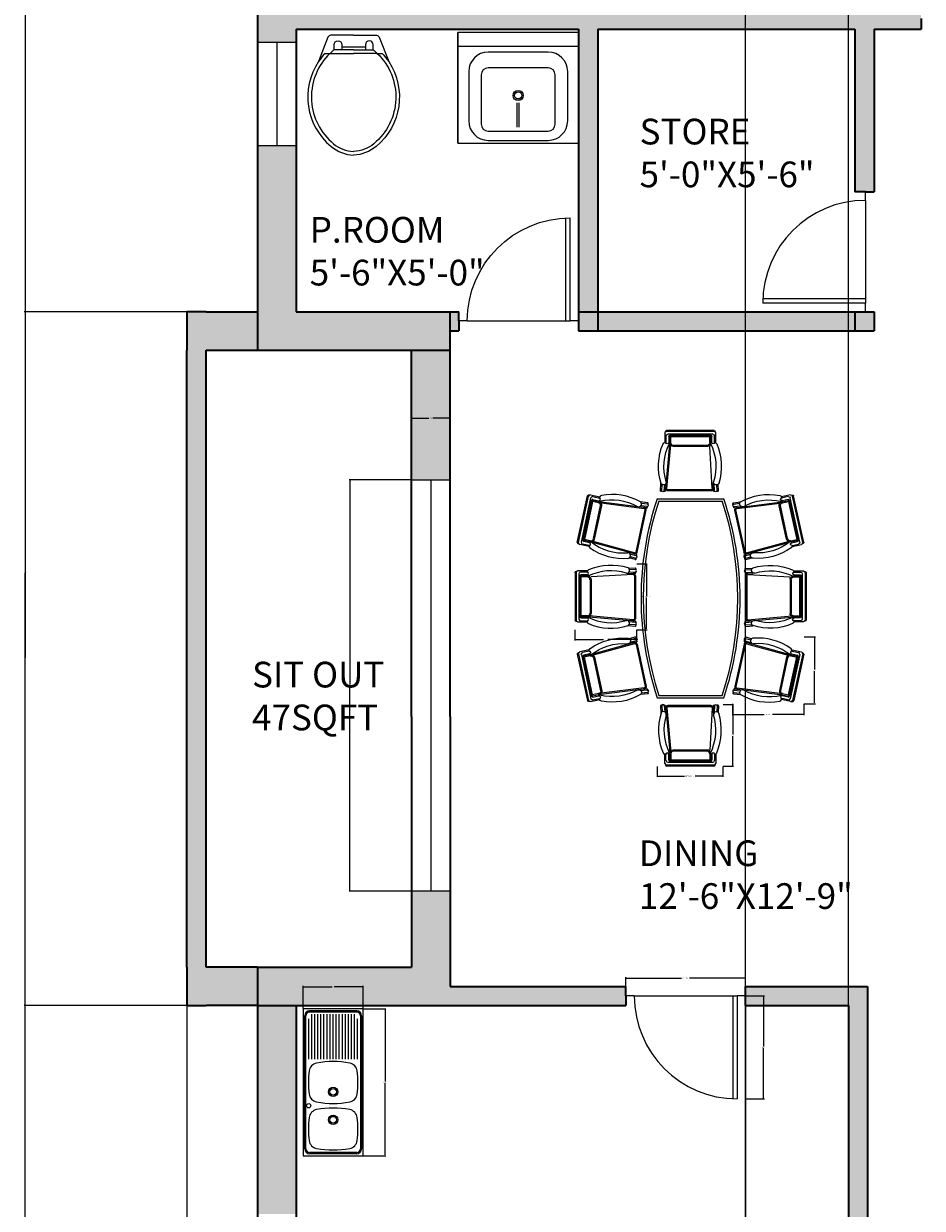
# Model space of a CAD drawing. Units: inches. Extents: x -36 to 442, y -676 to 151.
# Tile 3 of 8: x -36 to 174, y -411 to -134. Entities that reach past the tile are written whole.
import ezdxf

# ---------------------------------------------------------------- set-up
doc = ezdxf.new("R2010")
doc.units = ezdxf.units.IN
doc.header["$MEASUREMENT"] = 0
for name, color, linetype, lineweight in [('A-ANNO-DIMS', 2, 'Continuous', 18), ('A-AREA-IDEN', 7, 'Continuous', 18), ('A-DOOR', 4, 'Continuous', 18), ('A-FLOR-CASE', 32, 'Continuous', 18), ('A-FLOR-FIXT', 9, 'Continuous', 18), ('A-FURN', 9, 'Continuous', 13), ('A-GLAZ', 4, 'Continuous', 13), ('A-WALL', 7, 'Continuous', 35), ('A-WALL-PATT', 8, 'Continuous', 13), ('WC-Detail_dwgmodels.com', 251, 'Continuous', 13), ('WC-Outline_dwgmodels.com', 250, 'Continuous', 18)]:
    doc.layers.add(name, color=color, linetype=linetype, lineweight=lineweight)
doc.styles.get("Standard").update_dxf_attribs({"font": 'arial.ttf'})
doc.dimstyles.get("Standard").update_dxf_attribs({"dimtxt": 0.18, "dimasz": 0.18, "dimexe": 0.18, "dimexo": 0.0625, "dimgap": 0.09, "dimtad": 0, "dimtih": 1, "dimtoh": 1, "dimdec": 0, "dimzin": 0, "dimdsep": 46, "dimlunit": 3, "dimtxsty": 'Standard', "dimcen": 0.09, "dimadec": 0, "dimazin": 0, "dimtfac": 1, "dimtdec": 0, "dimtofl": 0, "dimtmove": 0, "dimatfit": 3, "dimfxl": 1, "dimtolj": 1, "dimtzin": 0, "dimarcsym": 0})

# ---------------------------------------------------------------- blocks, each defined once
blk = doc.blocks.new('М04 490х1200')
for p, q in [((-1200, 490), (-1200, 0)), ((0, 490), (-1200, 490)), ((0, 0), (0, 490)), ((-1183.5, 52.5), (-1183.5, 437.5)), ((-1173.5, 52.5), (-1173.5, 437.5)), ((-1143.5, 477.5), (-56.5, 477.5)), ((-1143.5, 467.5), (-56.5, 467.5)), ((-411, 445), (-80.8, 445)), ((-411, 420), (-45, 420)), ((-411, 395), (-45, 395)), ((-26.5, 52.5), (-26.5, 437.5)), ((-16.5, 52.5), (-16.5, 437.5)), ((-411, 370), (-45, 370)), ((-411, 345), (-45, 345)), ((-411, 320), (-45, 320)), ((-411, 295), (-45, 295)), ((-1173.5, 245), (-1173.5, 274.4)), ((-411, 270), (-45, 270)), ((-411, 245), (-45, 245)), ((-411, 220), (-45, 220)), ((-411, 195), (-45, 195)), ((-411, 170), (-45, 170)), ((-411, 145), (-45, 145)), ((-411, 120), (-45, 120)), ((-1200, 0), (0, 0)), ((-56.5, 22.5), (-1143.5, 22.5)), ((-56.5, 12.5), (-1143.5, 12.5)), ((-411, 95), (-45, 95)), ((-411, 70), (-45, 70)), ((-411, 45), (-82.9, 45))]:
    blk.add_line(p, q)
for centre, radius in [((-792, 445), 17.5), ((-906, 245), 38), ((-906, 245), 27.5), ((-678, 245), 38), ((-678, 245), 27.5)]:
    blk.add_circle(centre, radius)
for centre, radius, start, end in [((-1143.5, 437.5), 40, 90, 180), ((-1143.5, 437.5), 30, 90, 180), ((-1067, 366.6), 75, 97.23, 169.61876), ((-982, -303), 750, 82.77, 97.23), ((-897, 366.6), 75, 10.38124, 82.77), ((-687, 366.6), 75, 97.23, 169.61876), ((-602, -303), 750, 82.77, 97.23), ((-517, 366.6), 75, 10.38124, 82.77), ((-56.5, 437.5), 40, 0, 90), ((-56.5, 437.5), 30, 0, 90), ((-403, 245), 750, 169.61876, 190.38124), ((-1561, 245), 750, 349.61876, 10.38124), ((-23, 245), 750, 169.61876, 190.38124), ((-1181, 245), 750, 349.61876, 10.38124), ((-1067, 123.4), 75, 190.38124, 262.77), ((-897, 123.4), 75, 277.23, 349.61876), ((-687, 123.4), 75, 190.38124, 262.77), ((-517, 123.4), 75, 277.23, 349.61876), ((-1143.5, 52.5), 40, 180, 270), ((-1143.5, 52.5), 30, 180, 270), ((-982, 793), 750, 262.77, 277.23), ((-602, 793), 750, 262.77, 277.23), ((-56.5, 52.5), 30, 270, 0), ((-56.5, 52.5), 40, 270, 0)]:
    blk.add_arc(centre, radius, start, end)
blk = doc.blocks.new('М14 600х655')
for p, q in [((-655, 600), (-655, 0)), ((-655, 600), (-655, 0)), ((-655, 0), (-655, 600)), ((0, 600), (-655, 600)), ((0, 0), (0, 600)), ((0, 525), (-655, 525)), ((-165.1, 494.1), (-489.9, 494.1)), ((-595.8, 388.1), (-595.8, 121.3)), ((-165.4, 408.4), (-490.2, 408.4)), ((-59.2, 121.3), (-59.2, 388.1)), ((-528.4, 370.1), (-528.4, 103.3)), ((-127.2, 103.3), (-127.2, 370.1)), ((-333.5, 87.1), (-333.5, 219.6)), ((-321.5, 87.1), (-321.5, 219.6)), ((-490.2, 65.1), (-165.4, 65.1)), ((-655, 0), (-655, 0)), ((-655, 0), (-655, 0)), ((-655, 0), (0, 0)), ((-655, 0), (0, 0)), ((-489.9, 15.4), (-165.1, 15.4))]:
    blk.add_line(p, q)
for radius in [27.6, 19.3]:
    blk.add_circle((-327.5, 258.9), radius)
for centre, radius, start, end in [((-489.9, 388.1), 105.9, 90, 180), ((-165.1, 388.1), 105.9, 0, 90), ((-490.2, 370.1), 38.2, 90, 180), ((-165.4, 370.1), 38.2, 0, 90), ((-489.9, 121.3), 105.9, 180, 270), ((-490.2, 103.3), 38.2, 180, 270), ((-165.4, 103.3), 38.2, 270, 0), ((-165.1, 121.3), 105.9, 270, 0)]:
    blk.add_arc(centre, radius, start, end)
blk = doc.blocks.new('CHAIR-DINING-ANGLED')
for p, q in [((0.01, 4.02), (2.37, 14.86)), ((0.26, 3.97), (2.62, 14.8)), ((0.95, 4.08), (3.2, 14.41)), ((1.31, 4.53), (3.34, 13.85)), ((3.09, 15.1), (5.23, 14.63)), ((3.65, 14.05), (5.04, 13.75)), ((3.66, 14.71), (5.17, 14.38)), ((5.17, 14.39), (5.22, 14.59)), ((3.08, 12.46), (1.4, 4.76)), ((3.33, 12.4), (1.65, 4.7)), ((3.33, 13.6), (3.08, 12.46)), ((3.58, 13.55), (3.33, 12.4)), ((4.98, 13.24), (3.58, 13.55)), ((5.04, 13.5), (3.63, 13.8)), ((3.78, 4.9), (5.46, 12.61)), ((4.01, 4.75), (5.72, 12.55)), ((4.98, 13.24), (5.02, 13.23)), ((4.99, 13.76), (4.99, 13.76)), ((14.12, 12.35), (5.04, 13.5)), ((5.06, 13.49), (5.04, 13.49)), ((15.64, 11.9), (5.6, 13.16)), ((13.72, 1.76), (15.86, 11.59)), ((13.97, 1.71), (16.11, 11.54)), ((15.67, 12.16), (14.12, 12.35)), ((16.45, 13.28), (14.76, 13.47)), ((16.26, 12.42), (14.85, 12.58)), ((16.38, 12.97), (14.98, 13.14)), ((16.18, 12.09), (15.35, 12.2)), ((16.43, 12.99), (16.43, 12.99)), ((2.75, 3.03), (0.56, 3.51)), ((2.75, 3.29), (1.24, 3.62)), ((2.89, 3.92), (1.51, 4.22)), ((2.95, 4.15), (1.59, 4.45)), ((3.01, 4.4), (1.65, 4.7)), ((2.9, 3.92), (2.94, 4.13)), ((3.9, 3.93), (3.25, 4.12)), ((13.4, 1.57), (3.68, 4.26)), ((13.33, 1.32), (3.84, 3.95)), ((13.58, 0.01), (12.15, 0.41)), ((13.75, 0.89), (12.36, 1.28)), ((13.63, 0.34), (12.39, 0.68)), ((13.81, 1.19), (13.36, 1.32)), ((13.6, 0), (13.6, 0))]:
    blk.add_line(p, q)
for centre, radius, start, end in [((2.63, 14.81), 0.265, 57.0843, 167.6967), ((3, 14.72), 0.387, 77.6974, 167.697), ((3.58, 14.33), 0.387, 77.6974, 167.697), ((3.59, 13.8), 0.258, 77.6974, 167.697), ((5.1, 14.08), 0.326, 257.6968, 77.6966), ((8.15, 1.84), 12.09, 60.3857, 104.1301), ((5.72, 14.48), 0.516, 100.8762, 167.6967), ((8.15, 1.84), 13.38, 60.3857, 100.8762), ((3.58, 13.55), 0.258, 77.6967, 167.6967), ((4.96, 12.72), 0.516, 347.6967, 82.8716), ((5.24, 13.72), 0.207, 167.6967, 198.2858), ((5.16, 13.69), 0.129, 198.2858, 284.1301), ((4.96, 12.72), 0.774, 347.6967, 82.8716), ((14.35, 12.98), 0.644, 242.3299, 47.569), ((15.61, 11.65), 0.258, 347.6967, 82.8716), ((15.61, 11.65), 0.516, 347.6967, 82.8716), ((16.22, 12.26), 0.164, 256.5144, 76.5143), ((16.32, 12.69), 0.281, 257.6968, 77.6966), ((16.41, 13.12), 0.159, 257.6968, 77.6966), ((0.27, 3.98), 0.265, 167.6967, 257.6966), ((0.64, 3.88), 0.387, 167.697, 257.6967), ((1.32, 4), 0.387, 167.697, 257.6967), ((1.56, 4.48), 0.258, 167.697, 257.6967), ((1.65, 4.7), 0.258, 167.6967, 257.6967), ((3.25, 3.16), 0.516, 165.1864, 234.5172), ((2.8, 3.61), 0.326, 261.2909, 75.8056), ((3.07, 4.11), 0.129, 51.2332, 167.6967), ((3.15, 5.03), 0.645, 257.6967, 347.6967), ((10.72, 13.64), 12.09, 231.2332, 275.0077), ((3.26, 4.91), 0.774, 268.5122, 347.6967), ((10.72, 13.64), 13.38, 234.5172, 275.0077), ((11.81, 0.95, -7.02), 0.644, 273.0636, 93.0635), ((13.47, 1.82), 0.516, 254.5362, 347.6967), ((13.47, 1.82), 0.258, 254.5362, 347.6967), ((13.59, 0.18), 0.173, 256.4476, 76.4474), ((13.68, 0.63), 0.284, 257.6968, 77.6966), ((13.77, 1.05), 0.148, 256.2395, 76.2393)]:
    blk.add_arc(centre, radius, start, end)
blk = doc.blocks.new('CHAIR-DINING-SIDE')
for p, q in [((14.12, 14.02), (12.6, 13.93)), ((14.14, 14.02), (14.14, 14.02)), ((0.01, 12.98), (0.01, 1.89)), ((0.26, 12.98), (0.26, 1.89)), ((2.9, 13.37), (0.65, 13.37)), ((0.91, 12.73), (0.91, 2.15)), ((1.17, 12.21), (1.17, 2.67)), ((1.2, 2.91), (1.2, 11.97)), ((2.84, 13.11), (1.3, 13.11)), ((2.84, 12.47), (1.42, 12.47)), ((2.85, 12.23), (1.46, 12.23)), ((1.46, 2.91), (1.46, 11.97)), ((2.86, 11.97), (1.46, 11.97)), ((2.88, 13.11), (2.85, 13.11)), ((2.85, 12.46), (2.85, 12.25)), ((2.88, 12.45), (2.85, 12.45)), ((3.51, 11.33), (3.51, 3.43)), ((3.76, 11.42), (3.76, 3.43)), ((13.61, 12.53), (3.78, 11.98)), ((13.59, 12.78), (12.42, 12.72)), ((14.09, 13.11), (12.5, 13.02)), ((14.09, 13.68), (12.74, 13.61)), ((14.09, 12.81), (13.63, 12.78)), ((13.88, 12.27), (13.88, 2.21)), ((14.14, 12.27), (14.14, 2.21)), ((2.9, 2.91), (1.46, 2.91)), ((13.6, 1.95), (3.31, 2.88)), ((0.65, 1.51), (2.84, 1.51)), ((1.3, 1.76), (2.84, 1.76)), ((1.42, 2.41), (2.84, 2.41)), ((2.9, 2.66), (1.46, 2.66)), ((2.8, 2.41), (2.8, 2.41)), ((2.84, 1.76), (2.84, 1.55)), ((2.92, 2.66), (2.9, 2.66)), ((12.02, 1.84), (3.31, 2.62)), ((13.58, 1.7), (12.02, 1.84)), ((14.09, 0.44), (12.39, 0.59)), ((14.09, 0.76), (12.68, 0.88)), ((14.09, 1.32), (12.69, 1.46)), ((14.08, 1.65), (13.25, 1.72)), ((14.14, 0.72), (14.14, 0.72))]:
    blk.add_line(p, q)
for centre, radius, start, end in [((8.42, 1.31), 13.38, 72.689, 113.1795), ((12.09, 13.51), 0.659, 263.9479, 73.3079), ((14.1, 13.84), 0.173, 271.2493, 91.2491), ((0.27, 12.97), 0.265, 90.0001, 180), ((0.65, 12.98), 0.387, 90, 179.9996), ((1.3, 12.73), 0.387, 90, 179.9996), ((1.42, 12.21), 0.258, 90, 179.9996), ((1.46, 11.97), 0.258, 90, 180), ((2.83, 12.78), 0.315, 270.0001, 89.9999), ((3.36, 13.14), 0.516, 113.1795, 180), ((2.98, 12.25), 0.129, 180, 296.4635), ((2.86, 11.33), 0.645, 0, 90), ((8.42, 1.31), 12.09, 72.689, 116.4635), ((2.99, 11.42), 0.774, 0, 81.0504), ((13.62, 12.27), 0.516, 0, 93.1605), ((13.62, 12.27), 0.258, 0, 93.1605), ((14.08, 13.39), 0.284, 270.0001, 89.9999), ((14.09, 12.96), 0.148, 271.4574, 91.4572), ((1.46, 2.91), 0.258, 180, 270), ((2.99, 3.43), 0.774, 264.8251, 0), ((2.99, 3.43), 0.516, 264.8251, 0), ((0.27, 1.89), 0.265, 180, 269.9979), ((0.65, 1.89), 0.387, 179.9996, 269.9993), ((1.3, 2.15), 0.387, 179.9996, 269.9993), ((1.42, 2.67), 0.258, 179.9996, 269.9993), ((8.42, 13.38), 12.09, 242.2307, 242.4303), ((2.83, 2.07), 0.326, 270.0001, 89.9999), ((3.05, 2.4), 0.207, 149.4109, 180), ((3.36, 1.55), 0.516, 180, 246.8205), ((2.98, 2.44), 0.129, 63.5666, 149.4109), ((8.42, 13.38), 12.09, 243.5666, 287.311), ((8.42, 13.38), 13.38, 246.8205, 287.311), ((12.11, 1.17), 0.644, 285.3669, 105.3668), ((13.62, 2.21), 0.516, 264.8251, 0), ((13.62, 2.21), 0.258, 264.8251, 0), ((14.09, 1.48), 0.164, 271.1824, 91.1823), ((14.1, 1.04), 0.281, 270.0001, 89.9999), ((14.1, 0.6), 0.159, 270.0001, 89.9999)]:
    blk.add_arc(centre, radius, start, end)
blk = doc.blocks.new('CHAIR-DINING-END')
for p, q in [((0.44, 14.09), (0.59, 12.39)), ((0.72, 14.14), (0.72, 14.14)), ((0.76, 14.09), (0.88, 12.68)), ((1.32, 14.09), (1.46, 12.69)), ((1.65, 14.08), (1.73, 13.25)), ((12.27, 14.14), (2.21, 14.14)), ((12.27, 13.88), (2.21, 13.88)), ((12.81, 14.09), (12.78, 13.63)), ((13.11, 14.09), (13.02, 12.51)), ((13.68, 14.09), (13.61, 12.74)), ((14.02, 14.12), (13.93, 12.6)), ((14.02, 14.14), (14.02, 14.14)), ((1.7, 13.58), (2.63, 3.32)), ((1.95, 13.6), (2.88, 3.32)), ((12.53, 13.61), (11.98, 3.78)), ((12.78, 13.59), (12.72, 12.42)), ((1.51, 0.65), (1.51, 2.84)), ((1.76, 2.84), (1.55, 2.84)), ((1.76, 1.3), (1.76, 2.84)), ((2.41, 1.42), (2.41, 2.84)), ((2.41, 2.8), (2.41, 2.8)), ((2.66, 2.92), (2.66, 2.9)), ((2.66, 2.9), (2.66, 1.46)), ((2.92, 2.9), (2.92, 1.46)), ((11.42, 3.76), (3.43, 3.76)), ((11.33, 3.51), (3.43, 3.51)), ((11.97, 2.86), (11.97, 1.46)), ((12.23, 2.85), (12.23, 1.46)), ((12.46, 2.85), (12.25, 2.85)), ((12.45, 2.88), (12.45, 2.85)), ((12.47, 2.84), (12.47, 1.42)), ((13.11, 2.88), (13.11, 2.85)), ((13.11, 2.84), (13.11, 1.3)), ((13.37, 2.9), (13.37, 0.65)), ((12.98, 0.26), (1.89, 0.26)), ((12.98, 0.01), (1.89, 0.01)), ((12.73, 0.91), (2.15, 0.91)), ((12.21, 1.17), (2.67, 1.17)), ((2.92, 1.46), (11.97, 1.46)), ((2.92, 1.2), (11.97, 1.2))]:
    blk.add_line(p, q)
for centre, radius, start, end in [((0.6, 14.1), 0.159, 0.0001, 179.9999), ((1.04, 14.1), 0.281, 0.0001, 179.9999), ((1.48, 14.09), 0.164, 358.8177, 178.8176), ((2.21, 13.62), 0.516, 90, 185.1749), ((2.21, 13.62), 0.258, 90, 185.1749), ((12.27, 13.62), 0.516, 356.8395, 90), ((12.27, 13.62), 0.258, 356.8395, 90), ((12.96, 14.09), 0.148, 358.5428, 178.5426), ((13.39, 14.08), 0.284, 0.0001, 179.9999), ((13.84, 14.1), 0.173, 358.7509, 178.7507), ((13.38, 8.42), 13.38, 162.689, 203.1795), ((1.17, 12.11), 0.644, 344.6332, 164.6331), ((13.38, 8.42), 12.09, 162.689, 206.4334), ((1.31, 8.42), 12.09, 333.5365, 17.311), ((13.51, 12.09), 0.659, 16.6921, 186.0521), ((1.31, 8.42), 13.38, 336.8205, 17.311), ((1.55, 3.36), 0.516, 203.1795, 270), ((2.07, 2.83), 0.326, 0.0001, 179.9999), ((2.4, 3.05), 0.207, 270, 300.5891), ((2.44, 2.98), 0.129, 300.5891, 26.4334), ((3.43, 2.99), 0.774, 90, 185.1749), ((13.38, 8.42), 12.09, 207.5697, 207.7693), ((3.43, 2.99), 0.516, 90, 185.1749), ((11.33, 2.86), 0.645, 0, 90), ((11.42, 2.99), 0.774, 8.9496, 90), ((12.25, 2.98), 0.129, 153.5365, 270), ((12.78, 2.83), 0.315, 0.0001, 179.9999), ((13.14, 3.36), 0.516, 270, 336.8205), ((1.89, 0.65), 0.387, 180.0007, 270.0004), ((1.89, 0.27), 0.265, 180.0021, 270), ((2.15, 1.3), 0.387, 180.0007, 270.0004), ((2.67, 1.42), 0.258, 180.0007, 270.0004), ((2.92, 1.46), 0.258, 180, 270), ((11.97, 1.46), 0.258, 270, 0), ((12.21, 1.42), 0.258, 270.0004, 0), ((12.73, 1.3), 0.387, 270.0004, 0), ((12.97, 0.27), 0.265, 270, 359.9999), ((12.98, 0.65), 0.387, 270.0004, 0)]:
    blk.add_arc(centre, radius, start, end)
blk = doc.blocks.new('DOOR-SWING-24IN')
for p, q in [((24, 26), (24, 28)), ((24, 26), (24, 2)), ((24, 3), (0, 3)), ((24, 2), (0, 2)), ((24, 0), (24, 2))]:
    blk.add_line(p, q)
blk.add_arc((24, 2), 24, 90, 180)
blk = doc.blocks.new('GLAZING-UNIT-96IN')
for p, q in [((0, 0), (0, 96)), ((4.5, 96), (4.5, 0)), ((9, 96), (9, 0))]:
    blk.add_line(p, q)
blk = doc.blocks.new('*D17')
at = {"layer": 'A-ANNO-DIMS', "color": 0, "lineweight": -2, "transparency": 16777216}
for p, q in [((104.74, -361.18), (104.74, -356.87)), ((104.92, -357.05), (117.8, -357.05)), ((132.56, -357.05), (119.67, -357.05)), ((132.74, -361.18), (132.74, -356.87))]:
    blk.add_line(p, q, dxfattribs=at)
at = {"layer": 'A-ANNO-DIMS', "color": 0, "transparency": 16777216}
for points in [[(104.92, -357.02), (104.92, -357.08), (104.74, -357.05)], [(132.56, -357.02), (132.56, -357.08), (132.74, -357.05)]]:
    blk.add_solid(points, dxfattribs=at)
at = {"layer": 'Defpoints', "color": 0, "transparency": 16777216}
for p in [(104.74, -357.05), (104.74, -361.25), (132.74, -361.25)]:
    blk.add_point(p, dxfattribs=at)
at = {"layer": 'A-ANNO-DIMS', "color": 0, "transparency": 16777216, "insert": (118.74, -357.05), "char_height": 0.18, "attachment_point": 5}
blk.add_mtext('\\A1;DOOR 28 TYP.', dxfattribs=at)
blk = doc.blocks.new('*D18')
at = {"layer": 'A-ANNO-DIMS', "color": 0, "lineweight": -2, "transparency": 16777216}
for p, q in [((132.8, -361.25), (137.12, -361.25)), ((136.94, -361.43), (136.94, -373.07)), ((136.94, -385.07), (136.94, -373.43)), ((132.8, -385.25), (137.12, -385.25))]:
    blk.add_line(p, q, dxfattribs=at)
at = {"layer": 'A-ANNO-DIMS', "color": 0, "transparency": 16777216}
for points in [[(136.91, -361.43), (136.97, -361.43), (136.94, -361.25)], [(136.91, -385.07), (136.97, -385.07), (136.94, -385.25)]]:
    blk.add_solid(points, dxfattribs=at)
at = {"layer": 'Defpoints', "color": 0, "transparency": 16777216}
for p in [(132.74, -361.25), (136.94, -361.25), (132.74, -385.25)]:
    blk.add_point(p, dxfattribs=at)
at = {"layer": 'A-ANNO-DIMS', "color": 0, "transparency": 16777216, "insert": (136.94, -373.25), "char_height": 0.18, "attachment_point": 5}
blk.add_mtext('\\A1;24 TYP.', dxfattribs=at)
blk = doc.blocks.new('*D25')
at = {"layer": 'A-ANNO-DIMS', "color": 0, "lineweight": -2, "transparency": 16777216}
for p, q in [((54.67, -240.75), (40.16, -240.75)), ((40.34, -240.93), (40.34, -288.56)), ((40.34, -336.57), (40.34, -288.93)), ((54.67, -336.75), (40.16, -336.75))]:
    blk.add_line(p, q, dxfattribs=at)
at = {"layer": 'A-ANNO-DIMS', "color": 0, "transparency": 16777216}
for points in [[(40.31, -240.93), (40.37, -240.93), (40.34, -240.75)], [(40.31, -336.57), (40.37, -336.57), (40.34, -336.75)]]:
    blk.add_solid(points, dxfattribs=at)
at = {"layer": 'Defpoints', "color": 0, "transparency": 16777216}
for p in [(40.34, -240.75), (54.74, -240.75), (54.74, -336.75)]:
    blk.add_point(p, dxfattribs=at)
at = {"layer": 'A-ANNO-DIMS', "color": 0, "transparency": 16777216, "insert": (40.34, -288.75), "char_height": 0.18, "attachment_point": 5}
blk.add_mtext('\\A1;WINDOW 96 TYP.', dxfattribs=at)
blk = doc.blocks.new('*D26')
at = {"layer": 'A-ANNO-DIMS', "color": 0, "lineweight": -2, "transparency": 16777216}
for p, q in [((54.74, -240.68), (54.74, -226.17)), ((54.92, -226.35), (58.78, -226.35)), ((63.56, -226.35), (59.69, -226.35)), ((63.74, -240.68), (63.74, -226.17))]:
    blk.add_line(p, q, dxfattribs=at)
at = {"layer": 'A-ANNO-DIMS', "color": 0, "transparency": 16777216}
for points in [[(54.92, -226.32), (54.92, -226.38), (54.74, -226.35)], [(63.56, -226.32), (63.56, -226.38), (63.74, -226.35)]]:
    blk.add_solid(points, dxfattribs=at)
at = {"layer": 'Defpoints', "color": 0, "transparency": 16777216}
for p in [(63.74, -226.35), (54.74, -240.75), (63.74, -240.75)]:
    blk.add_point(p, dxfattribs=at)
at = {"layer": 'A-ANNO-DIMS', "color": 0, "transparency": 16777216, "insert": (59.24, -226.35), "char_height": 0.18, "attachment_point": 5}
blk.add_mtext('\\A1;9 TYP.', dxfattribs=at)
blk = doc.blocks.new('*D31')
at = {"layer": 'A-ANNO-DIMS', "color": 0, "lineweight": -2, "transparency": 16777216}
for p, q in [((43.48, -364.24), (48.74, -364.24)), ((48.56, -364.42), (48.56, -381.21)), ((48.56, -398.37), (48.56, -381.57)), ((43.48, -398.55), (48.74, -398.55))]:
    blk.add_line(p, q, dxfattribs=at)
at = {"layer": 'A-ANNO-DIMS', "color": 0, "transparency": 16777216}
for points in [[(48.53, -364.42), (48.59, -364.42), (48.56, -364.24)], [(48.53, -398.37), (48.59, -398.37), (48.56, -398.55)]]:
    blk.add_solid(points, dxfattribs=at)
at = {"layer": 'Defpoints', "color": 0, "transparency": 16777216}
for p in [(43.42, -364.24), (48.56, -364.24), (43.42, -398.55)]:
    blk.add_point(p, dxfattribs=at)
at = {"layer": 'A-ANNO-DIMS', "color": 0, "transparency": 16777216, "insert": (48.56, -381.39), "char_height": 0.18, "attachment_point": 5}
blk.add_mtext('\\A1;SINK 34', dxfattribs=at)
blk = doc.blocks.new('*D32')
at = {"layer": 'A-ANNO-DIMS', "color": 0, "lineweight": -2, "transparency": 16777216}
for p, q in [((29.41, -364.17), (29.41, -358.91)), ((29.59, -359.09), (36.2, -359.09)), ((43.24, -359.09), (36.62, -359.09)), ((43.42, -364.17), (43.42, -358.91))]:
    blk.add_line(p, q, dxfattribs=at)
at = {"layer": 'A-ANNO-DIMS', "color": 0, "transparency": 16777216}
for points in [[(29.59, -359.06), (29.59, -359.12), (29.41, -359.09)], [(43.24, -359.06), (43.24, -359.12), (43.42, -359.09)]]:
    blk.add_solid(points, dxfattribs=at)
at = {"layer": 'Defpoints', "color": 0, "transparency": 16777216}
for p in [(29.41, -359.09), (29.41, -364.24), (43.42, -364.24)]:
    blk.add_point(p, dxfattribs=at)
at = {"layer": 'A-ANNO-DIMS', "color": 0, "transparency": 16777216, "insert": (36.41, -359.09), "char_height": 0.18, "attachment_point": 5}
blk.add_mtext('\\A1;14', dxfattribs=at)
blk = doc.blocks.new('*D43')
at = {"layer": 'A-ANNO-DIMS', "color": 0, "lineweight": -2, "transparency": 16777216}
for p, q in [((107.33, -260.36), (109.75, -260.36)), ((109.57, -260.54), (109.57, -267.86)), ((109.57, -275.55), (109.57, -268.23)), ((107.33, -275.73), (109.75, -275.73))]:
    blk.add_line(p, q, dxfattribs=at)
at = {"layer": 'A-ANNO-DIMS', "color": 0, "transparency": 16777216}
for points in [[(109.54, -260.54), (109.6, -260.54), (109.57, -260.36)], [(109.54, -275.55), (109.6, -275.55), (109.57, -275.73)]]:
    blk.add_solid(points, dxfattribs=at)
at = {"layer": 'Defpoints', "color": 0, "transparency": 16777216}
for p in [(107.26, -260.36), (109.57, -260.36), (107.26, -275.73)]:
    blk.add_point(p, dxfattribs=at)
at = {"layer": 'A-ANNO-DIMS', "color": 0, "transparency": 16777216, "insert": (109.57, -268.05), "char_height": 0.18, "attachment_point": 5}
blk.add_mtext('\\A1;SIDE CHAIR 15 TYP.', dxfattribs=at)
blk = doc.blocks.new('*D44')
at = {"layer": 'A-ANNO-DIMS', "color": 0, "lineweight": -2, "transparency": 16777216}
for p, q in [((92.89, -275.8), (92.89, -278.22)), ((107.26, -275.8), (107.26, -278.22)), ((93.07, -278.04), (99.56, -278.04)), ((107.08, -278.04), (100.6, -278.04))]:
    blk.add_line(p, q, dxfattribs=at)
at = {"layer": 'A-ANNO-DIMS', "color": 0, "transparency": 16777216}
for points in [[(93.07, -278.01), (93.07, -278.07), (92.89, -278.04)], [(107.08, -278.01), (107.08, -278.07), (107.26, -278.04)]]:
    blk.add_solid(points, dxfattribs=at)
at = {"layer": 'Defpoints', "color": 0, "transparency": 16777216}
for p in [(92.89, -275.73), (107.26, -275.73), (107.26, -278.04)]:
    blk.add_point(p, dxfattribs=at)
at = {"layer": 'A-ANNO-DIMS', "color": 0, "transparency": 16777216, "insert": (100.08, -278.04), "char_height": 0.18, "attachment_point": 5}
blk.add_mtext('\\A1;14 TYP.', dxfattribs=at)
blk = doc.blocks.new('*D45')
at = {"layer": 'A-ANNO-DIMS', "color": 0, "lineweight": -2, "transparency": 16777216}
for p, q in [((112.05, -307.67), (112.05, -310.1)), ((127.42, -307.67), (127.42, -310.1)), ((112.23, -309.92), (118.48, -309.92)), ((127.24, -309.92), (120.98, -309.92))]:
    blk.add_line(p, q, dxfattribs=at)
at = {"layer": 'A-ANNO-DIMS', "color": 0, "transparency": 16777216}
for points in [[(112.23, -309.89), (112.23, -309.95), (112.05, -309.92)], [(127.24, -309.89), (127.24, -309.95), (127.42, -309.92)]]:
    blk.add_solid(points, dxfattribs=at)
at = {"layer": 'Defpoints', "color": 0, "transparency": 16777216}
for p in [(112.05, -307.61), (127.42, -307.61), (127.42, -309.92)]:
    blk.add_point(p, dxfattribs=at)
at = {"layer": 'A-ANNO-DIMS', "color": 0, "transparency": 16777216, "insert": (119.73, -309.92), "char_height": 0.18, "attachment_point": 5}
blk.add_mtext('\\A1;END CHAIR 15 TYP.', dxfattribs=at)
blk = doc.blocks.new('*D46')
at = {"layer": 'A-ANNO-DIMS', "color": 0, "lineweight": -2, "transparency": 16777216}
for p, q in [((127.48, -293.23), (129.91, -293.23)), ((129.73, -293.41), (129.73, -300.24)), ((129.73, -307.43), (129.73, -300.6)), ((127.48, -307.61), (129.91, -307.61))]:
    blk.add_line(p, q, dxfattribs=at)
at = {"layer": 'A-ANNO-DIMS', "color": 0, "transparency": 16777216}
for points in [[(129.7, -293.41), (129.76, -293.41), (129.73, -293.23)], [(129.7, -307.43), (129.76, -307.43), (129.73, -307.61)]]:
    blk.add_solid(points, dxfattribs=at)
at = {"layer": 'Defpoints', "color": 0, "transparency": 16777216}
for p in [(127.42, -293.23), (129.73, -293.23), (127.42, -307.61)]:
    blk.add_point(p, dxfattribs=at)
at = {"layer": 'A-ANNO-DIMS', "color": 0, "transparency": 16777216, "insert": (129.73, -300.42), "char_height": 0.18, "attachment_point": 5}
blk.add_mtext('\\A1;14 TYP.', dxfattribs=at)
blk = doc.blocks.new('*D47')
at = {"layer": 'A-ANNO-DIMS', "color": 0, "lineweight": -2, "transparency": 16777216}
for p, q in [((129.71, -293.07), (129.71, -295.69)), ((146.36, -293.07), (146.36, -295.69)), ((129.89, -295.51), (137.08, -295.51)), ((146.18, -295.51), (138.99, -295.51))]:
    blk.add_line(p, q, dxfattribs=at)
at = {"layer": 'A-ANNO-DIMS', "color": 0, "transparency": 16777216}
for points in [[(129.89, -295.48), (129.89, -295.54), (129.71, -295.51)], [(146.18, -295.48), (146.18, -295.54), (146.36, -295.51)]]:
    blk.add_solid(points, dxfattribs=at)
at = {"layer": 'Defpoints', "color": 0, "transparency": 16777216}
for p in [(129.71, -293.01), (146.36, -293.01), (129.71, -295.51)]:
    blk.add_point(p, dxfattribs=at)
at = {"layer": 'A-ANNO-DIMS', "color": 0, "transparency": 16777216, "insert": (138.04, -295.51), "char_height": 0.18, "attachment_point": 5}
blk.add_mtext('\\A1;CHAIR 17 TYP.', dxfattribs=at)
blk = doc.blocks.new('*D48')
at = {"layer": 'A-ANNO-DIMS', "color": 0, "lineweight": -2, "transparency": 16777216}
for p, q in [((146.43, -277.42), (149.04, -277.42)), ((148.86, -277.6), (148.86, -285.03)), ((148.86, -292.83), (148.86, -285.4)), ((146.43, -293.01), (149.04, -293.01))]:
    blk.add_line(p, q, dxfattribs=at)
at = {"layer": 'A-ANNO-DIMS', "color": 0, "transparency": 16777216}
for points in [[(148.83, -277.6), (148.89, -277.6), (148.86, -277.42)], [(148.83, -292.83), (148.89, -292.83), (148.86, -293.01)]]:
    blk.add_solid(points, dxfattribs=at)
at = {"layer": 'Defpoints', "color": 0, "transparency": 16777216}
for p in [(146.36, -277.42), (146.36, -293.01), (148.86, -293.01)]:
    blk.add_point(p, dxfattribs=at)
at = {"layer": 'A-ANNO-DIMS', "color": 0, "transparency": 16777216, "insert": (148.86, -285.21), "char_height": 0.18, "attachment_point": 5}
blk.add_mtext('\\A1;16 TYP.', dxfattribs=at)
blk = doc.blocks.new('*D49')
at = {"layer": 'A-ANNO-DIMS', "color": 0, "lineweight": -2, "transparency": 16777216}
for p, q in [((2.24, -363.56), (2.24, -675.98)), ((404.24, -512.06), (404.24, -675.98)), ((2.42, -675.8), (202.94, -675.8)), ((404.06, -675.8), (203.53, -675.8))]:
    blk.add_line(p, q, dxfattribs=at)
at = {"layer": 'A-ANNO-DIMS', "color": 0, "transparency": 16777216}
for points in [[(2.42, -675.77), (2.42, -675.83), (2.24, -675.8)], [(404.06, -675.77), (404.06, -675.83), (404.24, -675.8)]]:
    blk.add_solid(points, dxfattribs=at)
at = {"layer": 'Defpoints', "color": 0, "transparency": 16777216}
for p in [(2.24, -363.5), (404.24, -512), (404.24, -675.8)]:
    blk.add_point(p, dxfattribs=at)
at = {"layer": 'A-ANNO-DIMS', "color": 0, "transparency": 16777216, "insert": (203.24, -675.8), "char_height": 0.18, "attachment_point": 5}
blk.add_mtext('\\A1;402', dxfattribs=at)
blk = doc.blocks.new('*D50')
at = {"layer": 'A-ANNO-DIMS', "color": 0, "lineweight": -2, "transparency": 16777216}
for p, q in [((97.44, 113.5), (-35.74, 113.5)), ((-35.56, 113.32), (-35.56, -262.07)), ((-35.56, -637.82), (-35.56, -262.43)), ((18.67, -638), (-35.74, -638))]:
    blk.add_line(p, q, dxfattribs=at)
at = {"layer": 'A-ANNO-DIMS', "color": 0, "transparency": 16777216}
for points in [[(-35.59, 113.32), (-35.53, 113.32), (-35.56, 113.5)], [(-35.59, -637.82), (-35.53, -637.82), (-35.56, -638)]]:
    blk.add_solid(points, dxfattribs=at)
at = {"layer": 'Defpoints', "color": 0, "transparency": 16777216}
for p in [(-35.56, 113.5), (97.5, 113.5), (18.74, -638)]:
    blk.add_point(p, dxfattribs=at)
at = {"layer": 'A-ANNO-DIMS', "color": 0, "transparency": 16777216, "insert": (-35.56, -262.25), "char_height": 0.18, "attachment_point": 5}
blk.add_mtext('\\A1;751.5', dxfattribs=at)
blk = doc.blocks.new('*D54')
at = {"layer": 'A-ANNO-DIMS', "color": 0, "lineweight": -2, "transparency": 16777216}
for p, q in [((2.17, -201.5), (-35.74, -201.5)), ((-35.56, -201.68), (-35.56, -282.32)), ((-35.56, -363.32), (-35.56, -282.68)), ((2.17, -363.5), (-35.74, -363.5))]:
    blk.add_line(p, q, dxfattribs=at)
at = {"layer": 'A-ANNO-DIMS', "color": 0, "transparency": 16777216}
for points in [[(-35.59, -201.68), (-35.53, -201.68), (-35.56, -201.5)], [(-35.59, -363.32), (-35.53, -363.32), (-35.56, -363.5)]]:
    blk.add_solid(points, dxfattribs=at)
at = {"layer": 'Defpoints', "color": 0, "transparency": 16777216}
for p in [(2.24, -201.5), (-35.56, -363.5), (2.24, -363.5)]:
    blk.add_point(p, dxfattribs=at)
at = {"layer": 'A-ANNO-DIMS', "color": 0, "transparency": 16777216, "insert": (-35.56, -282.5), "char_height": 0.18, "attachment_point": 5}
blk.add_mtext('\\A1;162', dxfattribs=at)
blk = doc.blocks.new('*D63')
at = {"layer": 'A-ANNO-DIMS', "color": 0, "lineweight": -2, "transparency": 16777216}
for p, q in [((132.74, -447.43), (132.74, 151.48)), ((132.92, 151.3), (144.51, 151.3)), ((156.56, 151.3), (144.96, 151.3)), ((156.74, -471.43), (156.74, 151.48))]:
    blk.add_line(p, q, dxfattribs=at)
at = {"layer": 'A-ANNO-DIMS', "color": 0, "transparency": 16777216}
for points in [[(132.92, 151.33), (132.92, 151.27), (132.74, 151.3)], [(156.56, 151.33), (156.56, 151.27), (156.74, 151.3)]]:
    blk.add_solid(points, dxfattribs=at)
at = {"layer": 'Defpoints', "color": 0, "transparency": 16777216}
for p in [(156.74, 151.3), (132.74, -447.5), (156.74, -471.5)]:
    blk.add_point(p, dxfattribs=at)
at = {"layer": 'A-ANNO-DIMS', "color": 0, "transparency": 16777216, "insert": (144.74, 151.3), "char_height": 0.18, "attachment_point": 5}
blk.add_mtext('\\A1;24', dxfattribs=at)

msp = doc.modelspace()

# ---------------------------------------------------------------- hatches: boundary and pattern name
at = {"layer": 'A-WALL-PATT'}
h = msp.add_hatch(color=256, dxfattribs=at)
h.dxf.hatch_style = 1
h.paths.add_polyline_path([(288, 113.503), (193.5, 113.503), (97.5, 113.503), (97.5, 104.864), (106.5, 104.864), (106.5, 104.503), (193.5, 104.503), (193.5, 5.503), (193.5, 1.003), (213.735, 1.003), (213.735, -135.497), (218.235, -135.497), (218.235, 1.003), (251, 1.003), (251, 3.253), (251, 5.503), (198, 5.503), (198, 104.503), (279, 104.503), (279, 104.209), (288, 104.209)])
h.paths.add_polyline_path([(378.735, 81.646), (362.235, 81.646), (288, 81.646), (288, 80.209), (279, 80.209), (279, 5.503), (279, 1.003), (353.235, 1.003), (353.235, 0.242), (362.235, 0.242), (362.235, 5.503), (288, 5.503), (288, 77.146), (362.235, 77.146), (374.235, 77.146), (374.235, 5.503), (362.235, 5.503), (362.235, 1.003), (374.235, 1.003), (378.735, 1.003), (378.735, 5.503), (378.735, 77.146)])
h.paths.add_polyline_path([(362.235, -35.758), (353.235, -35.758), (353.235, -196.997), (218.235, -196.997), (213.735, -196.997), (213.735, -205.997), (218.235, -205.997), (378.735, -205.997), (378.735, -205.779), (387.735, -205.779), (387.735, -202.472), (387.735, -196.997), (378.735, -196.997), (362.235, -196.997)])
h.paths.add_polyline_path([(218.235, -175.497), (215.985, -175.497), (213.735, -175.497), (213.735, -196.997), (218.235, -196.997)], flags=17)
h.paths.add_polyline_path([(158.235, -201.497), (98.235, -201.497), (98.235, -205.997), (158.235, -205.997)])
h.paths.add_polyline_path([(173.735, -130.997), (27.735, -130.997), (27.735, -35.267), (18.735, -35.267), (18.735, -138.68), (27.735, -138.68), (27.735, -135.497), (93.735, -135.497), (93.735, -201.497), (98.235, -201.497), (98.235, -135.497), (158.235, -135.497), (158.235, -173.497), (160.739, -173.497), (162.735, -173.497), (162.735, -135.497), (173.735, -135.497), (173.735, -133.017)])
h.paths.add_polyline_path([(98.235, -201.497), (93.735, -201.497), (93.735, -205.997), (98.235, -205.997)])
h.paths.add_polyline_path([(162.735, -201.497), (158.235, -201.497), (158.235, -205.997), (162.735, -205.997)])
h.paths.add_polyline_path([(63.735, -205.997), (63.735, -201.497), (27.735, -201.497), (27.735, -162.68), (18.735, -162.68), (18.735, -210.497), (63.735, -210.497)])
h.paths.add_polyline_path([(65.735, -203.604), (65.735, -201.497), (63.735, -201.497), (63.735, -205.997), (65.735, -205.997)])
h.paths.add_polyline_path([(165.5, 5.503), (106.5, 5.503), (106.5, 80.864), (97.5, 80.864), (97.5, 81.646), (6.735, 81.646), (2.235, 81.646), (2.235, 77.146), (2.235, 5.503), (2.235, 1.003), (6.735, 1.003), (18.735, 1.003), (18.735, 5.503), (6.735, 5.503), (6.735, 77.146), (97.5, 77.146), (97.5, 5.503), (18.735, 5.503), (18.735, 0.733), (27.735, 0.733), (27.735, 1.003), (165.5, 1.003), (165.5, 3.253)])
h.paths.add_polyline_path([(18.735, -201.497), (6.735, -201.497), (2.235, -201.497), (2.235, -210.497), (2.235, -354.497), (2.235, -363.497), (6.735, -363.497), (18.735, -363.497), (18.735, -358.997), (18.735, -354.497), (6.735, -354.497), (6.735, -210.497), (18.735, -210.497)])
h.paths.add_polyline_path([(63.735, -210.497), (54.735, -210.497), (54.735, -240.747), (63.735, -240.747)])
h.paths.add_polyline_path([(63.735, -336.747), (54.735, -336.747), (54.735, -354.497), (18.735, -354.497), (18.735, -358.997), (18.735, -363.497), (104.735, -363.497), (104.735, -361.247), (104.735, -358.997), (63.735, -358.997)])
h.paths.add_polyline_path([(27.735, -448.151), (18.735, -448.151), (18.735, -637.997), (72.735, -637.997), (72.735, -571.997), (183.235, -571.997), (183.235, -562.997), (57.197, -562.997), (51.735, -562.997), (51.735, -567.497), (57.197, -567.497), (63.735, -567.497), (63.735, -571.997), (63.735, -628.997), (27.735, -628.997), (27.735, -475.997), (27.735, -471.497)])
h.paths.add_polyline_path([(27.735, -363.497), (18.735, -363.497), (18.735, -412.151), (27.735, -412.151)])
h.paths.add_polyline_path([(161.235, -358.997), (132.735, -358.997), (132.735, -363.497), (156.735, -363.497), (156.735, -471.497), (51.735, -471.497), (51.735, -475.997), (63.735, -475.997), (63.735, -534.997), (65.985, -534.997), (68.235, -534.997), (68.235, -475.997), (161.235, -475.997)])
h.paths.add_polyline_path([(161.235, -511.997), (173.235, -511.997), (173.235, -502.997), (161.235, -502.997), (161.235, -475.997), (152.235, -475.997), (152.235, -534.997), (156.735, -534.997), (161.235, -534.997)], flags=17)
h.paths.add_polyline_path([(362.235, -502.997), (353.235, -502.997), (213.235, -502.997), (213.235, -507.497), (213.235, -511.997), (362.235, -511.997)])
h.paths.add_polyline_path([(242.235, -548.019), (233.235, -548.019), (233.235, -562.997), (223.235, -562.997), (223.235, -567.497), (223.235, -571.997), (242.235, -571.997)])
h.paths.add_polyline_path([(404.235, -502.997), (399.735, -502.997), (362.235, -502.997), (362.235, -511.997), (399.735, -511.997), (404.235, -511.997)])
h.paths.add_polyline_path([(362.235, -482.123), (353.235, -482.123), (353.235, -502.997), (362.235, -502.997)])
h.paths.add_polyline_path([(404.235, -295.997), (404.235, -286.997), (387.735, -286.997), (387.735, -295.997), (399.735, -295.997), (399.735, -502.997), (404.235, -502.997)])
h.paths.add_polyline_path([(362.235, -355.863), (353.235, -355.863), (353.235, -386.123), (362.235, -386.123)])
h.paths.add_polyline_path([(387.735, -286.997), (378.735, -286.997), (213.735, -286.997), (213.735, -295.997), (353.235, -295.997), (353.235, -295.863), (362.235, -295.863), (362.235, -295.997), (378.735, -295.997), (387.735, -295.997)])
h.paths.add_polyline_path([(387.735, -241.779), (378.735, -241.779), (378.735, -286.997), (387.735, -286.997)])
h.paths.add_polyline_path([(387.735, -175.497), (362.235, -175.497), (362.235, -184.497), (387.735, -184.497)], flags=17)
h.paths.add_polyline_path([(387.735, -184.497), (383.235, -184.497), (383.235, -192.497), (378.735, -192.497), (366.735, -192.497), (366.735, -184.497), (362.235, -184.497), (362.235, -196.997), (378.735, -196.997), (387.735, -196.997)], flags=17)
h.paths.add_polyline_path([(240.604, 40.967), (282.575, 40.967), (282.575, 63.356), (240.604, 63.356)], flags=25)

# ---------------------------------------------------------------- linework, layer by layer
at = {"layer": 'A-FLOR-CASE'}
msp.add_line((132.735, -363.497), (132.735, -446.014), dxfattribs=at)
at = {"layer": 'A-FURN'}
for p, q in [((112.067, -245.185), (127.664, -245.185)), ((112.44, -245.701), (127.292, -245.701)), ((112.108, -291.614), (127.66, -291.614)), ((112.48, -291.098), (127.287, -291.098))]:
    msp.add_line(p, q, dxfattribs=at)
for centre, radius, start, end in [((181.738, -268.338), 73.418, 161.61728, 198.48347), ((181.738, -268.338), 72.902, 161.90954, 198.19175), ((58.367, -268.393), 72.564, 341.76615, 18.22322), ((58.367, -268.393), 73.08, 341.4733, 18.51612)]:
    msp.add_arc(centre, radius, start, end, dxfattribs=at)
at = {"layer": 'A-GLAZ'}
for p, q in [((18.735, -138.68), (18.735, -162.68)), ((27.735, -138.68), (18.735, -138.68)), ((23.235, -138.68), (23.235, -162.68)), ((27.735, -162.68), (27.735, -138.68)), ((18.735, -162.68), (27.735, -162.68)), ((54.735, -240.747), (63.735, -240.747)), ((63.735, -336.747), (54.735, -336.747))]:
    msp.add_line(p, q, dxfattribs=at)
at = {"layer": 'A-WALL'}
for p, q in [((18.735, 5.503), (18.735, -210.497)), ((27.735, -135.497), (93.735, -135.497)), ((27.735, -135.497), (27.735, -201.497)), ((93.735, -135.497), (93.735, -205.997)), ((98.235, -135.497), (98.235, -205.997)), ((98.235, -135.497), (158.235, -135.497)), ((158.235, -135.497), (158.235, -173.497)), ((162.735, -135.497), (162.735, -173.497)), ((162.735, -135.497), (173.735, -135.497)), ((173.735, -133.017), (173.735, -135.497)), ((160.739, -173.497), (158.235, -173.497)), ((160.739, -173.497), (162.735, -173.497)), ((6.735, -201.497), (2.235, -201.497)), ((2.235, -201.497), (2.235, -210.497)), ((6.735, -201.497), (18.735, -201.497)), ((27.735, -201.497), (65.735, -201.497)), ((63.735, -205.997), (63.735, -201.497)), ((65.735, -203.604), (65.735, -201.497)), ((93.735, -201.497), (162.735, -201.497)), ((158.235, -201.497), (158.235, -205.997)), ((162.735, -201.497), (162.735, -205.997)), ((65.735, -203.604), (65.735, -205.997)), ((63.735, -205.997), (65.735, -205.997)), ((63.735, -295.997), (63.735, -205.997)), ((93.735, -205.997), (162.735, -205.997)), ((2.235, -354.497), (2.235, -210.497)), ((6.735, -354.497), (6.735, -210.497)), ((6.735, -210.497), (18.735, -210.497)), ((18.735, -210.497), (63.735, -210.497)), ((54.735, -295.997), (54.735, -210.497)), ((54.735, -295.997), (54.735, -354.497)), ((63.735, -295.997), (63.735, -358.997)), ((2.235, -354.497), (2.235, -363.497)), ((18.735, -354.497), (6.735, -354.497)), ((18.735, -354.497), (54.735, -354.497)), ((18.735, -354.497), (18.735, -358.997)), ((18.735, -358.997), (18.735, -637.997)), ((63.735, -358.997), (104.735, -358.997)), ((104.735, -361.247), (104.735, -358.997)), ((132.735, -363.497), (132.735, -358.997)), ((132.735, -358.997), (161.235, -358.997)), ((161.235, -358.997), (161.235, -502.997)), ((104.735, -361.247), (104.735, -363.497)), ((2.235, -363.497), (6.735, -363.497)), ((18.735, -363.497), (6.735, -363.497)), ((18.735, -363.497), (104.735, -363.497)), ((27.735, -363.497), (27.735, -471.497)), ((132.735, -363.497), (156.735, -363.497)), ((156.735, -363.497), (156.735, -471.497))]:
    msp.add_line(p, q, dxfattribs=at)
at = {"layer": 'WC-Detail_dwgmodels.com'}
for p, q in [((34.51, -141.182), (35.685, -141.182)), ((46.698, -141.182), (47.872, -141.182))]:
    msp.add_line(p, q, dxfattribs=at)
for points in [[(36.65, -140.337), (36.65, -139.162, -1), (38.435, -139.162), (38.435, -139.773)], [(45.733, -140.337), (45.733, -139.162, 1), (43.947, -139.162), (43.947, -139.773)], [(36.65, -140.337, 0.0227116), (35.685, -141.182, 0.1626183)], [(41.191, -140.337), (36.65, -140.337, 0.0227116)], [(41.191, -140.337), (45.733, -140.337, -0.4761076)], [(45.733, -140.337, -0.0227116), (46.698, -141.182, -0.1626183)], [(34.51, -141.182, 0.0409366), (32.995, -143.103, 0.1637323)], [(47.872, -141.182, -0.0409366), (49.388, -143.103, -0.1637323)]]:
    msp.add_lwpolyline(points, format="xyb", dxfattribs=at)
for points in [[(43.947, -139.773), (38.435, -139.773)], [(38.435, -139.773), (38.435, -140.337)], [(43.947, -139.773), (43.947, -140.337)]]:
    msp.add_lwpolyline(points, dxfattribs=at)
at = {"layer": 'WC-Outline_dwgmodels.com'}
for p in [(35.685, -141.182), (46.698, -141.182)]:
    msp.add_line(p, (41.191, -141.182), dxfattribs=at)
for points in [[(41.191, -136.944), (35.846, -136.944, 0.3103103), (35.191, -137.394), (32.995, -143.103, 0.2090713)], [(41.191, -136.944), (46.536, -136.944, -0.3103103), (47.192, -137.394), (49.388, -143.103, -0.2090713)], [(32.995, -143.103, 0.3839185), (35.93, -162.918, 0.1637323), (41.191, -164.935, 0.3597326)], [(35.123, -141.752, 0.4316389), (36.463, -162.273, 0.1626183), (41.191, -164.098, 0.4708774)], [(35.685, -141.182, 0.0141645), (35.123, -141.752, 0.1626183)], [(46.698, -141.182, -0.4485458), (45.92, -162.273, -0.1626183), (41.191, -164.098, -0.4708774)], [(49.388, -143.103, -0.3839185), (46.453, -162.918, -0.1637323), (41.191, -164.935, -0.3597326)]]:
    msp.add_lwpolyline(points, format="xyb", dxfattribs=at)

# ---------------------------------------------------------------- block references
at = {"layer": 'A-DOOR'}
msp.add_blockref('DOOR-SWING-24IN', (136.739, -201.497), dxfattribs=at)
at = {"layer": 'A-DOOR', "extrusion": (0, 0, -1), "zscale": -1, "rotation": 270.0000000000005}
msp.add_blockref('DOOR-SWING-24IN', (-93.735, -179.604), dxfattribs=at)
at = {"layer": 'A-DOOR', "rotation": 90.00000000000063}
msp.add_blockref('DOOR-SWING-24IN', (132.735, -385.247), dxfattribs=at)
at = {"layer": 'A-FLOR-FIXT', "xscale": 0.0430748895547816, "yscale": 0.0430748895547816, "zscale": 0.0430748895547816}
msp.add_blockref('М14 600х655', (93.735, -162.159), dxfattribs=at)
at = {"layer": 'A-FLOR-FIXT', "xscale": 0.0285919858329957, "yscale": 0.0285919858329957, "zscale": 0.0285919858329957, "rotation": 90}
msp.add_blockref('М04 490х1200', (43.416, -364.235), dxfattribs=at)
at = {"layer": 'A-FURN', "extrusion": (0, 0, -1), "zscale": -1}
for name, p, rotation in [('CHAIR-DINING-END', (-112.388, -229.196), 180), ('CHAIR-DINING-ANGLED', (-146.337, -259.369), 359.9851397709624), ('CHAIR-DINING-ANGLED', (-93.429, -277.427), 180)]:
    msp.add_blockref(name, p, dxfattribs=dict(at, rotation=rotation))
at = {"layer": 'A-FURN'}
for name, p in [('CHAIR-DINING-ANGLED', (93.429, -259.379)), ('CHAIR-DINING-SIDE', (92.888, -275.392)), ('CHAIR-DINING-END', (112.388, -307.61))]:
    msp.add_blockref(name, p, dxfattribs=at)
at = {"layer": 'A-FURN', "extrusion": (0, 0, -1), "zscale": -1}
msp.add_blockref('CHAIR-DINING-SIDE', (-146.88, -275.392), dxfattribs=at)
at = {"layer": 'A-FURN', "rotation": 180}
msp.add_blockref('CHAIR-DINING-ANGLED', (146.339, -277.427), dxfattribs=at)
at = {"layer": 'A-GLAZ'}
msp.add_blockref('GLAZING-UNIT-96IN', (54.735, -336.746), dxfattribs=at)

# ---------------------------------------------------------------- texts
at = {"layer": 'A-AREA-IDEN', "char_height": 6, "attachment_point": 1}
for s, insert in [('STORE\\P5\'-0"X5\'-6"', (107.981, -156.444)), ('P.ROOM\\P5\'-6"X5\'-0"', (30.937, -179.37)), ('SIT OUT\\P47SQFT', (17.473, -283.221)), ('DINING\\P12\'-6"X12\'-9"', (107.83, -324.925))]:
    msp.add_mtext(s, dxfattribs=dict(at, insert=insert))

# ---------------------------------------------------------------- dimensions: what is measured, and where the dimension line sits
at = {"layer": 'A-ANNO-DIMS'}
for base, p1, p2, picture, middle in [((156.735, 151.303), (132.735, -447.497), (156.735, -471.497), '*D63', (144.735, 151.303)), ((404.235, -675.797), (2.235, -363.497), (404.235, -511.997), '*D49', (203.235, -675.797))]:
    dim = msp.add_linear_dim(base=base, p1=p1, p2=p2, dimstyle='Standard', override={"dimdec": 0, "dimlfac": 1, "dimrnd": 0, "dimzin": 0, "dimdsep": 46, "dimlunit": 2}, dxfattribs=at)
    dim.commit()
    dim.dimension.update_dxf_attribs({"geometry": picture, "text_midpoint": middle})
for base, p1, p2, angle, override, picture, middle in [((-35.565, 113.503), (18.735, -637.997), (97.5, 113.503), 90, {"dimdec": 1, "dimlfac": 1, "dimrnd": 0, "dimzin": 0, "dimdsep": 46, "dimlunit": 2}, '*D50', (-35.565, -262.247)), ((-35.565, -363.497), (2.235, -201.497), (2.235, -363.497), 90, {"dimdec": 0, "dimlfac": 1, "dimrnd": 0, "dimzin": 0, "dimdsep": 46, "dimlunit": 2}, '*D54', (-35.565, -282.497)), ((29.405, -359.089), (43.416, -364.235), (29.405, -364.235), 180, {"dimdec": 0, "dimlfac": 1, "dimrnd": 0, "dimzin": 0, "dimdsep": 46, "dimlunit": 2}, '*D32', (36.411, -359.089))]:
    dim = msp.add_linear_dim(base=base, p1=p1, p2=p2, angle=angle, dimstyle='Standard', override=override, dxfattribs=at)
    dim.commit()
    dim.dimension.update_dxf_attribs({"geometry": picture, "text_midpoint": middle})
for base, p1, p2, text, picture, middle in [((63.735, -226.347), (54.735, -240.747), (63.735, -240.747), '<> TYP.', '*D26', (59.235, -226.347)), ((107.264, -278.041), (92.888, -275.735), (107.264, -275.735), '<> TYP.', '*D44', (100.076, -278.041)), ((127.421, -309.916), (112.046, -307.61), (127.421, -307.61), 'END CHAIR <> TYP.', '*D45', (119.733, -309.916))]:
    dim = msp.add_linear_dim(base=base, p1=p1, p2=p2, text=text, dimstyle='Standard', override={"dimdec": 0, "dimlfac": 1, "dimrnd": 0, "dimzin": 0, "dimdsep": 46, "dimlunit": 2}, dxfattribs=at)
    dim.commit()
    dim.dimension.update_dxf_attribs({"geometry": picture, "text_midpoint": middle})
for base, p1, p2, angle, text, picture, middle in [((40.335, -240.747), (54.735, -336.747), (54.735, -240.747), 90, 'WINDOW <> TYP.', '*D25', (40.335, -288.747)), ((109.57, -260.36), (107.264, -275.735), (107.264, -260.36), 90, 'SIDE CHAIR <> TYP.', '*D43', (109.57, -268.047)), ((148.862, -293.01), (146.364, -277.42), (146.364, -293.01), 270, '<> TYP.', '*D48', (148.862, -285.215)), ((129.711, -295.508), (146.364, -293.01), (129.711, -293.01), 180, 'CHAIR <> TYP.', '*D47', (138.037, -295.508)), ((129.727, -293.234), (127.421, -307.61), (127.421, -293.234), 90, '<> TYP.', '*D46', (129.727, -300.422)), ((104.735, -357.047), (132.735, -361.247), (104.735, -361.247), 180, 'DOOR <> TYP.', '*D17', (118.735, -357.047)), ((136.935, -361.247), (132.735, -385.247), (132.735, -361.247), 90, '<> TYP.', '*D18', (136.935, -373.247)), ((48.562, -364.235), (43.416, -398.546), (43.416, -364.235), 90, 'SINK <>', '*D31', (48.562, -381.391))]:
    dim = msp.add_linear_dim(base=base, p1=p1, p2=p2, angle=angle, text=text, dimstyle='Standard', override={"dimdec": 0, "dimlfac": 1, "dimrnd": 0, "dimzin": 0, "dimdsep": 46, "dimlunit": 2}, dxfattribs=at)
    dim.commit()
    dim.dimension.update_dxf_attribs({"geometry": picture, "text_midpoint": middle})

doc.saveas('drawing.dxf')
